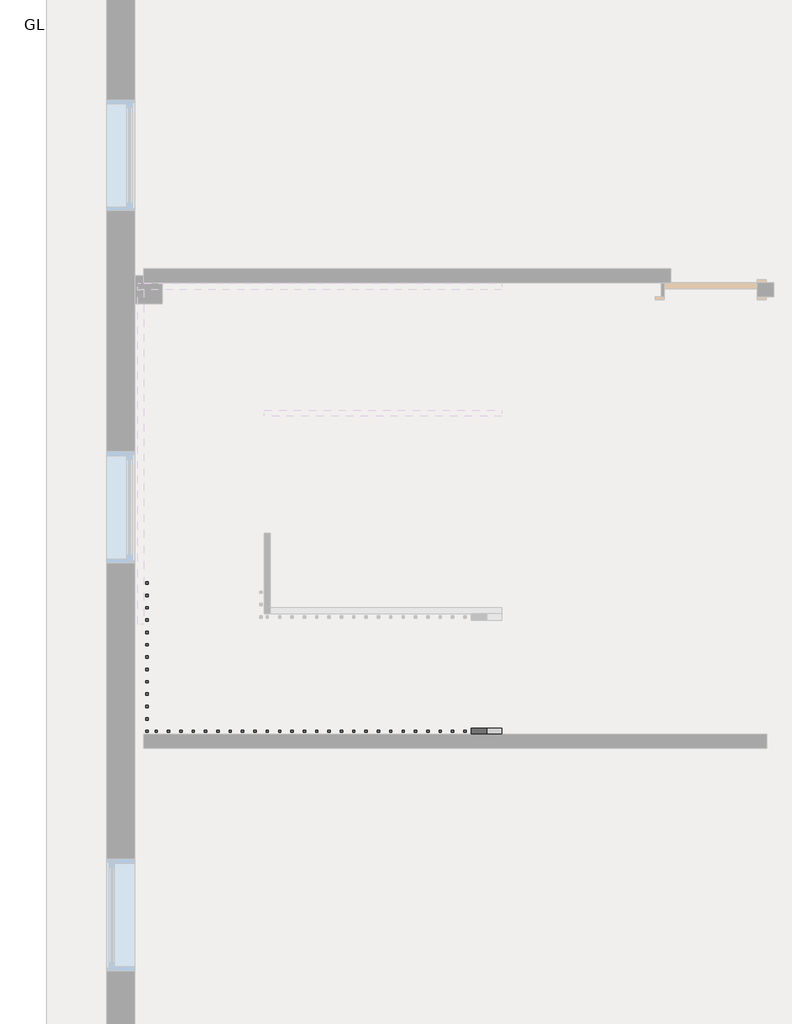
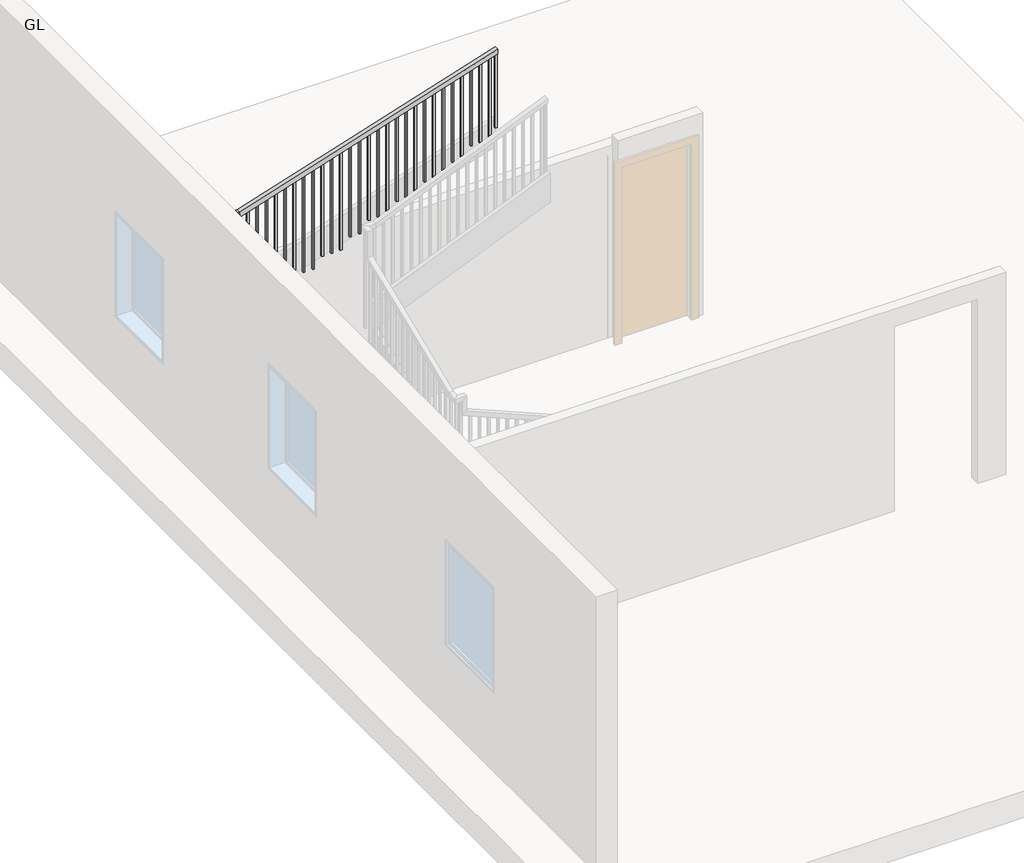
# One storey, part 2 of 3: 1 railing.
"""IFC4 building model written with IfcOpenShell, lengths in millimetres."""

from ifc_helpers import new_model, si_unit, frame, origin, place, context, project, spatial, polyline, outline, extrude, faceted_brep, element, save

model = new_model("IFC4")

# Units and contexts
model_context = context("Model", 3, world=origin())
ifc_project = project(units=[si_unit("LENGTHUNIT", "METRE", prefix="MILLI")], contexts=[model_context])

# Site, building, storey
site = spatial("IfcSite", under=ifc_project)
building = spatial("IfcBuilding", under=site)
storey = spatial("IfcBuildingStorey", under=building, Name="GL", Elevation=3200.4)

# Railing
placement = place(None, origin())
element("IfcRailing", 1, ObjectType="Handrail - Rectangular", at=placement, inside=storey, context=model_context, shape_type="SolidModel", body=[
    faceted_brep([(5202.3334712, 4110.8450307, 4349.2615385), (5202.3334712, 4110.8450307, 4294.1711054), (5202.3334712, 4161.6450307, 4294.1711054), (5202.3334712, 4161.6450307, 4349.2615385), (2978.1401378, 4110.8450307, 5282.4895105), (2967.9146058, 4110.8450307, 5231.6895105), (2967.9146058, 4161.6450307, 5231.6895105), (2978.1401378, 4161.6450307, 5282.4895105), (2255.9334712, 4110.8450307, 5231.6895105), (2255.9334712, 4110.8450307, 5282.4895105), (2255.9334712, 5086.4359398, 5282.4895105), (2255.9334712, 5094.0746153, 5231.6895105), (2306.7334712, 4161.6450307, 5231.6895105), (2306.7334712, 5094.0746153, 5231.6895105), (2306.7334712, 4161.6450307, 5282.4895105), (2306.7334712, 5086.4359398, 5282.4895105), (5202.3334712, 7768.4450307, 7045.5692308), (5202.3334712, 7717.6450307, 7045.5692308), (5202.3334712, 7717.6450307, 6992.2578701), (5202.3334712, 7768.4450307, 6992.2578701), (2390.8233294, 7768.4450307, 6097.3474801), (2382.9334712, 7768.4450307, 6148.1474801), (2390.8233294, 7717.6450307, 6097.3474801), (2382.9334712, 7717.6450307, 6148.1474801), (2255.9334712, 7641.4450307, 6068.6461538), (2255.9334712, 7692.2450307, 6031.1265614), (2306.7334712, 7692.2450307, 6031.1265614), (2306.7334712, 7641.4450307, 6068.6461538), (2255.9334712, 7641.4450307, 6148.1474801), (2255.9334712, 7692.2450307, 6097.3474801), (2306.7334712, 7692.2450307, 6097.3474801), (2306.7334712, 7641.4450307, 6148.1474801), (2255.9334712, 7768.4450307, 6148.1474801), (2255.9334712, 7768.4450307, 6097.3474801), (2306.7334712, 7717.6450307, 6097.3474801), (2306.7334712, 7717.6450307, 6148.1474801)], [[[0, 1, 2, 3]], [[1, 0, 4, 5]], [[2, 1, 5, 6]], [[3, 2, 6, 7]], [[0, 3, 7, 4]], [[8, 9, 10, 11]], [[12, 8, 11, 13]], [[14, 12, 13, 15]], [[9, 14, 15, 10]], [[16, 17, 18, 19]], [[20, 21, 16, 19]], [[22, 20, 19, 18]], [[23, 22, 18, 17]], [[21, 23, 17, 16]], [[5, 4, 9, 8]], [[6, 5, 8, 12]], [[7, 6, 12, 14]], [[4, 7, 14, 9]], [[11, 10, 24, 25]], [[13, 11, 25, 26]], [[15, 13, 26, 27]], [[10, 15, 27, 24]], [[25, 24, 28, 29]], [[26, 25, 29, 30]], [[27, 26, 30, 31]], [[24, 27, 31, 28]], [[29, 28, 32, 33]], [[30, 29, 33, 34]], [[31, 30, 34, 35]], [[28, 31, 35, 32]], [[33, 32, 21, 20]], [[34, 33, 20, 22]], [[35, 34, 22, 23]], [[32, 35, 23, 21]]]),
    extrude(outline(polyline([(6964.9713979, 5116.6084712), (6013.9384615, 5116.6084712), (6013.9384615, 5135.6584712), (6971.0350584, 5135.6584712), (6964.9713979, 5116.6084712)])), frame((0.0, 7733.5200307, 0.0), z_axis=(0.0, 1.0, 0.0), x_axis=(0.0, 0.0, 1.0)), (0.0, 0.0, 1.0), 19.05),
    extrude(outline(polyline([(6932.6318754, 5015.0084712), (6013.9384615, 5015.0084712), (6013.9384615, 5034.0584712), (6938.6955359, 5034.0584712), (6932.6318754, 5015.0084712)])), frame((0.0, 7733.5200307, 0.0), z_axis=(0.0, 1.0, 0.0), x_axis=(0.0, 0.0, 1.0)), (0.0, 0.0, 1.0), 19.05),
    extrude(outline(polyline([(6900.2923528, 4913.4084712), (6013.9384615, 4913.4084712), (6013.9384615, 4932.4584712), (6906.3560133, 4932.4584712), (6900.2923528, 4913.4084712)])), frame((0.0, 7733.5200307, 0.0), z_axis=(0.0, 1.0, 0.0), x_axis=(0.0, 0.0, 1.0)), (0.0, 0.0, 1.0), 19.05),
    extrude(outline(polyline([(6867.9528303, 4811.8084712), (5896.7076923, 4811.8084712), (5896.7076923, 4830.8584712), (6874.0164908, 4830.8584712), (6867.9528303, 4811.8084712)])), frame((0.0, 7733.5200307, 0.0), z_axis=(0.0, 1.0, 0.0), x_axis=(0.0, 0.0, 1.0)), (0.0, 0.0, 1.0), 19.05),
    extrude(outline(polyline([(6835.6133077, 4710.2084712), (5896.7076923, 4710.2084712), (5896.7076923, 4729.2584712), (6841.6769682, 4729.2584712), (6835.6133077, 4710.2084712)])), frame((0.0, 7733.5200307, 0.0), z_axis=(0.0, 1.0, 0.0), x_axis=(0.0, 0.0, 1.0)), (0.0, 0.0, 1.0), 19.05),
    extrude(outline(polyline([(6803.2737852, 4608.6084712), (5779.4769231, 4608.6084712), (5779.4769231, 4627.6584712), (6809.3374457, 4627.6584712), (6803.2737852, 4608.6084712)])), frame((0.0, 7733.5200307, 0.0), z_axis=(0.0, 1.0, 0.0), x_axis=(0.0, 0.0, 1.0)), (0.0, 0.0, 1.0), 19.05),
    extrude(outline(polyline([(6770.9342626, 4507.0084712), (5779.4769231, 4507.0084712), (5779.4769231, 4526.0584712), (6776.9979231, 4526.0584712), (6770.9342626, 4507.0084712)])), frame((0.0, 7733.5200307, 0.0), z_axis=(0.0, 1.0, 0.0), x_axis=(0.0, 0.0, 1.0)), (0.0, 0.0, 1.0), 19.05),
    extrude(outline(polyline([(6738.5947401, 4405.4084712), (5779.4769231, 4405.4084712), (5779.4769231, 4424.4584712), (6744.6584006, 4424.4584712), (6738.5947401, 4405.4084712)])), frame((0.0, 7733.5200307, 0.0), z_axis=(0.0, 1.0, 0.0), x_axis=(0.0, 0.0, 1.0)), (0.0, 0.0, 1.0), 19.05),
    extrude(outline(polyline([(6706.2552176, 4303.8084712), (5662.2461538, 4303.8084712), (5662.2461538, 4322.8584712), (6712.318878, 4322.8584712), (6706.2552176, 4303.8084712)])), frame((0.0, 7733.5200307, 0.0), z_axis=(0.0, 1.0, 0.0), x_axis=(0.0, 0.0, 1.0)), (0.0, 0.0, 1.0), 19.05),
    extrude(outline(polyline([(6673.915695, 4202.2084712), (5662.2461538, 4202.2084712), (5662.2461538, 4221.2584712), (6679.9793555, 4221.2584712), (6673.915695, 4202.2084712)])), frame((0.0, 7733.5200307, 0.0), z_axis=(0.0, 1.0, 0.0), x_axis=(0.0, 0.0, 1.0)), (0.0, 0.0, 1.0), 19.05),
    extrude(outline(polyline([(6641.5761725, 4100.6084712), (5662.2461538, 4100.6084712), (5662.2461538, 4119.6584712), (6647.6398329, 4119.6584712), (6641.5761725, 4100.6084712)])), frame((0.0, 7733.5200307, 0.0), z_axis=(0.0, 1.0, 0.0), x_axis=(0.0, 0.0, 1.0)), (0.0, 0.0, 1.0), 19.05),
    extrude(outline(polyline([(6609.2366499, 3999.0084712), (5545.0153846, 3999.0084712), (5545.0153846, 4018.0584712), (6615.3003104, 4018.0584712), (6609.2366499, 3999.0084712)])), frame((0.0, 7733.5200307, 0.0), z_axis=(0.0, 1.0, 0.0), x_axis=(0.0, 0.0, 1.0)), (0.0, 0.0, 1.0), 19.05),
    extrude(outline(polyline([(6576.8971274, 3897.4084712), (5545.0153846, 3897.4084712), (5545.0153846, 3916.4584712), (6582.9607878, 3916.4584712), (6576.8971274, 3897.4084712)])), frame((0.0, 7733.5200307, 0.0), z_axis=(0.0, 1.0, 0.0), x_axis=(0.0, 0.0, 1.0)), (0.0, 0.0, 1.0), 19.05),
    extrude(outline(polyline([(6544.5576048, 3795.8084712), (5545.0153846, 3795.8084712), (5545.0153846, 3814.8584712), (6550.6212653, 3814.8584712), (6544.5576048, 3795.8084712)])), frame((0.0, 7733.5200307, 0.0), z_axis=(0.0, 1.0, 0.0), x_axis=(0.0, 0.0, 1.0)), (0.0, 0.0, 1.0), 19.05),
    extrude(outline(polyline([(6512.2180823, 3694.2084712), (5427.7846154, 3694.2084712), (5427.7846154, 3713.2584712), (6518.2817427, 3713.2584712), (6512.2180823, 3694.2084712)])), frame((0.0, 7733.5200307, 0.0), z_axis=(0.0, 1.0, 0.0), x_axis=(0.0, 0.0, 1.0)), (0.0, 0.0, 1.0), 19.05),
    extrude(outline(polyline([(6479.8785597, 3592.6084712), (5427.7846154, 3592.6084712), (5427.7846154, 3611.6584712), (6485.9422202, 3611.6584712), (6479.8785597, 3592.6084712)])), frame((0.0, 7733.5200307, 0.0), z_axis=(0.0, 1.0, 0.0), x_axis=(0.0, 0.0, 1.0)), (0.0, 0.0, 1.0), 19.05),
    extrude(outline(polyline([(6447.5390372, 3491.0084712), (5310.5538462, 3491.0084712), (5310.5538462, 3510.0584712), (6453.6026977, 3510.0584712), (6447.5390372, 3491.0084712)])), frame((0.0, 7733.5200307, 0.0), z_axis=(0.0, 1.0, 0.0), x_axis=(0.0, 0.0, 1.0)), (0.0, 0.0, 1.0), 19.05),
    extrude(outline(polyline([(6415.1995146, 3389.4084712), (5310.5538462, 3389.4084712), (5310.5538462, 3408.4584712), (6421.2631751, 3408.4584712), (6415.1995146, 3389.4084712)])), frame((0.0, 7733.5200307, 0.0), z_axis=(0.0, 1.0, 0.0), x_axis=(0.0, 0.0, 1.0)), (0.0, 0.0, 1.0), 19.05),
    extrude(outline(polyline([(6382.8599921, 3287.8084712), (5310.5538462, 3287.8084712), (5310.5538462, 3306.8584712), (6388.9236526, 3306.8584712), (6382.8599921, 3287.8084712)])), frame((0.0, 7733.5200307, 0.0), z_axis=(0.0, 1.0, 0.0), x_axis=(0.0, 0.0, 1.0)), (0.0, 0.0, 1.0), 19.05),
    extrude(outline(polyline([(6350.5204695, 3186.2084712), (5193.3230769, 3186.2084712), (5193.3230769, 3205.2584712), (6356.58413, 3205.2584712), (6350.5204695, 3186.2084712)])), frame((0.0, 7733.5200307, 0.0), z_axis=(0.0, 1.0, 0.0), x_axis=(0.0, 0.0, 1.0)), (0.0, 0.0, 1.0), 19.05),
    extrude(outline(polyline([(6318.180947, 3084.6084712), (5193.3230769, 3084.6084712), (5193.3230769, 3103.6584712), (6324.2446075, 3103.6584712), (6318.180947, 3084.6084712)])), frame((0.0, 7733.5200307, 0.0), z_axis=(0.0, 1.0, 0.0), x_axis=(0.0, 0.0, 1.0)), (0.0, 0.0, 1.0), 19.05),
    extrude(outline(polyline([(6285.8414244, 2983.0084712), (5193.3230769, 2983.0084712), (5193.3230769, 3002.0584712), (6291.9050849, 3002.0584712), (6285.8414244, 2983.0084712)])), frame((0.0, 7733.5200307, 0.0), z_axis=(0.0, 1.0, 0.0), x_axis=(0.0, 0.0, 1.0)), (0.0, 0.0, 1.0), 19.05),
    extrude(outline(polyline([(6253.5019019, 2881.4084712), (5193.3230769, 2881.4084712), (5193.3230769, 2900.4584712), (6259.5655624, 2900.4584712), (6253.5019019, 2881.4084712)])), frame((0.0, 7733.5200307, 0.0), z_axis=(0.0, 1.0, 0.0), x_axis=(0.0, 0.0, 1.0)), (0.0, 0.0, 1.0), 19.05),
    extrude(outline(polyline([(6221.1623794, 2779.8084712), (5193.3230769, 2779.8084712), (5193.3230769, 2798.8584712), (6227.2260398, 2798.8584712), (6221.1623794, 2779.8084712)])), frame((0.0, 7733.5200307, 0.0), z_axis=(0.0, 1.0, 0.0), x_axis=(0.0, 0.0, 1.0)), (0.0, 0.0, 1.0), 19.05),
    extrude(outline(polyline([(6188.8228568, 2678.2084712), (5193.3230769, 2678.2084712), (5193.3230769, 2697.2584712), (6194.8865173, 2697.2584712), (6188.8228568, 2678.2084712)])), frame((0.0, 7733.5200307, 0.0), z_axis=(0.0, 1.0, 0.0), x_axis=(0.0, 0.0, 1.0)), (0.0, 0.0, 1.0), 19.05),
    extrude(outline(polyline([(6156.4833343, 2576.6084712), (5193.3230769, 2576.6084712), (5193.3230769, 2595.6584712), (6162.5469947, 2595.6584712), (6156.4833343, 2576.6084712)])), frame((0.0, 7733.5200307, 0.0), z_axis=(0.0, 1.0, 0.0), x_axis=(0.0, 0.0, 1.0)), (0.0, 0.0, 1.0), 19.05),
    extrude(outline(polyline([(6124.1438117, 2475.0084712), (5193.3230769, 2475.0084712), (5193.3230769, 2494.0584712), (6130.2074722, 2494.0584712), (6124.1438117, 2475.0084712)])), frame((0.0, 7733.5200307, 0.0), z_axis=(0.0, 1.0, 0.0), x_axis=(0.0, 0.0, 1.0)), (0.0, 0.0, 1.0), 19.05),
    extrude(outline(polyline([(6091.8042892, 2373.4084712), (5193.3230769, 2373.4084712), (5193.3230769, 2392.4584712), (6097.8679496, 2392.4584712), (6091.8042892, 2373.4084712)])), frame((0.0, 7733.5200307, 0.0), z_axis=(0.0, 1.0, 0.0), x_axis=(0.0, 0.0, 1.0)), (0.0, 0.0, 1.0), 19.05),
    extrude(outline(polyline([(2271.8084712, 7682.7200307), (2271.8084712, 7701.7700307), (2290.8584712, 7701.7700307), (2290.8584712, 7682.7200307), (2271.8084712, 7682.7200307)])), frame((0.0, 0.0, 5076.0923077), z_axis=(0.0, 0.0, 1.0), x_axis=(1.0, 0.0, 0.0)), (0.0, 0.0, 1.0), 1021.2551724),
    extrude(outline(polyline([(7600.1700307, 6002.7957922), (7600.1700307, 5076.0923077), (7581.1200307, 5076.0923077), (7581.1200307, 5996.9342537), (7600.1700307, 6002.7957922)])), frame((2271.8084712, 0.0, 0.0), z_axis=(1.0, 0.0, 0.0), x_axis=(0.0, 1.0, 0.0)), (0.0, 0.0, 1.0), 19.05),
    extrude(outline(polyline([(7498.5700307, 5971.5342537), (7498.5700307, 5076.0923077), (7479.5200307, 5076.0923077), (7479.5200307, 5965.6727152), (7498.5700307, 5971.5342537)])), frame((2271.8084712, 0.0, 0.0), z_axis=(1.0, 0.0, 0.0), x_axis=(0.0, 1.0, 0.0)), (0.0, 0.0, 1.0), 19.05),
    extrude(outline(polyline([(7396.9700307, 5940.2727152), (7396.9700307, 5076.0923077), (7377.9200307, 5076.0923077), (7377.9200307, 5934.4111768), (7396.9700307, 5940.2727152)])), frame((2271.8084712, 0.0, 0.0), z_axis=(1.0, 0.0, 0.0), x_axis=(0.0, 1.0, 0.0)), (0.0, 0.0, 1.0), 19.05),
    extrude(outline(polyline([(7295.3700307, 5909.0111768), (7295.3700307, 5076.0923077), (7276.3200307, 5076.0923077), (7276.3200307, 5903.1496383), (7295.3700307, 5909.0111768)])), frame((2271.8084712, 0.0, 0.0), z_axis=(1.0, 0.0, 0.0), x_axis=(0.0, 1.0, 0.0)), (0.0, 0.0, 1.0), 19.05),
    extrude(outline(polyline([(7193.7700307, 5877.7496383), (7193.7700307, 5076.0923077), (7174.7200307, 5076.0923077), (7174.7200307, 5871.8880999), (7193.7700307, 5877.7496383)])), frame((2271.8084712, 0.0, 0.0), z_axis=(1.0, 0.0, 0.0), x_axis=(0.0, 1.0, 0.0)), (0.0, 0.0, 1.0), 19.05),
    extrude(outline(polyline([(7092.1700307, 5846.4880999), (7092.1700307, 5076.0923077), (7073.1200307, 5076.0923077), (7073.1200307, 5840.6265614), (7092.1700307, 5846.4880999)])), frame((2271.8084712, 0.0, 0.0), z_axis=(1.0, 0.0, 0.0), x_axis=(0.0, 1.0, 0.0)), (0.0, 0.0, 1.0), 19.05),
    extrude(outline(polyline([(6990.5700307, 5815.2265614), (6990.5700307, 5076.0923077), (6971.5200307, 5076.0923077), (6971.5200307, 5809.3650229), (6990.5700307, 5815.2265614)])), frame((2271.8084712, 0.0, 0.0), z_axis=(1.0, 0.0, 0.0), x_axis=(0.0, 1.0, 0.0)), (0.0, 0.0, 1.0), 19.05),
    extrude(outline(polyline([(6888.9700307, 5783.9650229), (6888.9700307, 5076.0923077), (6869.9200307, 5076.0923077), (6869.9200307, 5778.1034845), (6888.9700307, 5783.9650229)])), frame((2271.8084712, 0.0, 0.0), z_axis=(1.0, 0.0, 0.0), x_axis=(0.0, 1.0, 0.0)), (0.0, 0.0, 1.0), 19.05),
    extrude(outline(polyline([(6787.3700307, 5752.7034845), (6787.3700307, 5076.0923077), (6768.3200307, 5076.0923077), (6768.3200307, 5746.841946), (6787.3700307, 5752.7034845)])), frame((2271.8084712, 0.0, 0.0), z_axis=(1.0, 0.0, 0.0), x_axis=(0.0, 1.0, 0.0)), (0.0, 0.0, 1.0), 19.05),
    extrude(outline(polyline([(6685.7700307, 5721.441946), (6685.7700307, 4958.8615385), (6666.7200307, 4958.8615385), (6666.7200307, 5715.5804076), (6685.7700307, 5721.441946)])), frame((2271.8084712, 0.0, 0.0), z_axis=(1.0, 0.0, 0.0), x_axis=(0.0, 1.0, 0.0)), (0.0, 0.0, 1.0), 19.05),
    extrude(outline(polyline([(6584.1700307, 5690.1804076), (6584.1700307, 4958.8615385), (6565.1200307, 4958.8615385), (6565.1200307, 5684.3188691), (6584.1700307, 5690.1804076)])), frame((2271.8084712, 0.0, 0.0), z_axis=(1.0, 0.0, 0.0), x_axis=(0.0, 1.0, 0.0)), (0.0, 0.0, 1.0), 19.05),
    extrude(outline(polyline([(6482.5700307, 5658.9188691), (6482.5700307, 4841.6307692), (6463.5200307, 4841.6307692), (6463.5200307, 5653.0573306), (6482.5700307, 5658.9188691)])), frame((2271.8084712, 0.0, 0.0), z_axis=(1.0, 0.0, 0.0), x_axis=(0.0, 1.0, 0.0)), (0.0, 0.0, 1.0), 19.05),
    extrude(outline(polyline([(6380.9700307, 5627.6573306), (6380.9700307, 4841.6307692), (6361.9200307, 4841.6307692), (6361.9200307, 5621.7957922), (6380.9700307, 5627.6573306)])), frame((2271.8084712, 0.0, 0.0), z_axis=(1.0, 0.0, 0.0), x_axis=(0.0, 1.0, 0.0)), (0.0, 0.0, 1.0), 19.05),
    extrude(outline(polyline([(6279.3700307, 5596.3957922), (6279.3700307, 4841.6307692), (6260.3200307, 4841.6307692), (6260.3200307, 5590.5342537), (6279.3700307, 5596.3957922)])), frame((2271.8084712, 0.0, 0.0), z_axis=(1.0, 0.0, 0.0), x_axis=(0.0, 1.0, 0.0)), (0.0, 0.0, 1.0), 19.05),
    extrude(outline(polyline([(6177.7700307, 5565.1342537), (6177.7700307, 4724.4), (6158.7200307, 4724.4), (6158.7200307, 5559.2727152), (6177.7700307, 5565.1342537)])), frame((2271.8084712, 0.0, 0.0), z_axis=(1.0, 0.0, 0.0), x_axis=(0.0, 1.0, 0.0)), (0.0, 0.0, 1.0), 19.05),
    extrude(outline(polyline([(6076.1700307, 5533.8727152), (6076.1700307, 4724.4), (6057.1200307, 4724.4), (6057.1200307, 5528.0111768), (6076.1700307, 5533.8727152)])), frame((2271.8084712, 0.0, 0.0), z_axis=(1.0, 0.0, 0.0), x_axis=(0.0, 1.0, 0.0)), (0.0, 0.0, 1.0), 19.05),
    extrude(outline(polyline([(5974.5700307, 5502.6111768), (5974.5700307, 4724.4), (5955.5200307, 4724.4), (5955.5200307, 5496.7496383), (5974.5700307, 5502.6111768)])), frame((2271.8084712, 0.0, 0.0), z_axis=(1.0, 0.0, 0.0), x_axis=(0.0, 1.0, 0.0)), (0.0, 0.0, 1.0), 19.05),
    extrude(outline(polyline([(5872.9700307, 5471.3496383), (5872.9700307, 4607.1692308), (5853.9200307, 4607.1692308), (5853.9200307, 5465.4880999), (5872.9700307, 5471.3496383)])), frame((2271.8084712, 0.0, 0.0), z_axis=(1.0, 0.0, 0.0), x_axis=(0.0, 1.0, 0.0)), (0.0, 0.0, 1.0), 19.05),
    extrude(outline(polyline([(5771.3700307, 5440.0880999), (5771.3700307, 4607.1692308), (5752.3200307, 4607.1692308), (5752.3200307, 5434.2265614), (5771.3700307, 5440.0880999)])), frame((2271.8084712, 0.0, 0.0), z_axis=(1.0, 0.0, 0.0), x_axis=(0.0, 1.0, 0.0)), (0.0, 0.0, 1.0), 19.05),
    extrude(outline(polyline([(5669.7700307, 5408.8265614), (5669.7700307, 4607.1692308), (5650.7200307, 4607.1692308), (5650.7200307, 5402.9650229), (5669.7700307, 5408.8265614)])), frame((2271.8084712, 0.0, 0.0), z_axis=(1.0, 0.0, 0.0), x_axis=(0.0, 1.0, 0.0)), (0.0, 0.0, 1.0), 19.05),
    extrude(outline(polyline([(5568.1700307, 5377.5650229), (5568.1700307, 4489.9384615), (5549.1200307, 4489.9384615), (5549.1200307, 5371.7034845), (5568.1700307, 5377.5650229)])), frame((2271.8084712, 0.0, 0.0), z_axis=(1.0, 0.0, 0.0), x_axis=(0.0, 1.0, 0.0)), (0.0, 0.0, 1.0), 19.05),
    extrude(outline(polyline([(5466.5700307, 5346.3034845), (5466.5700307, 4489.9384615), (5447.5200307, 4489.9384615), (5447.5200307, 5340.441946), (5466.5700307, 5346.3034845)])), frame((2271.8084712, 0.0, 0.0), z_axis=(1.0, 0.0, 0.0), x_axis=(0.0, 1.0, 0.0)), (0.0, 0.0, 1.0), 19.05),
    extrude(outline(polyline([(5364.9700307, 5315.041946), (5364.9700307, 4372.7076923), (5345.9200307, 4372.7076923), (5345.9200307, 5309.1804076), (5364.9700307, 5315.041946)])), frame((2271.8084712, 0.0, 0.0), z_axis=(1.0, 0.0, 0.0), x_axis=(0.0, 1.0, 0.0)), (0.0, 0.0, 1.0), 19.05),
    extrude(outline(polyline([(5263.3700307, 5283.7804076), (5263.3700307, 4372.7076923), (5244.3200307, 4372.7076923), (5244.3200307, 5277.9188691), (5263.3700307, 5283.7804076)])), frame((2271.8084712, 0.0, 0.0), z_axis=(1.0, 0.0, 0.0), x_axis=(0.0, 1.0, 0.0)), (0.0, 0.0, 1.0), 19.05),
    extrude(outline(polyline([(5161.7700307, 5252.5188691), (5161.7700307, 4372.7076923), (5142.7200307, 4372.7076923), (5142.7200307, 5246.6573306), (5161.7700307, 5252.5188691)])), frame((2271.8084712, 0.0, 0.0), z_axis=(1.0, 0.0, 0.0), x_axis=(0.0, 1.0, 0.0)), (0.0, 0.0, 1.0), 19.05),
    extrude(outline(polyline([(2271.8084712, 5041.1200307), (2271.8084712, 5060.1700307), (2290.8584712, 5060.1700307), (2290.8584712, 5041.1200307), (2271.8084712, 5041.1200307)])), frame((0.0, 0.0, 4255.4769231), z_axis=(0.0, 0.0, 1.0), x_axis=(1.0, 0.0, 0.0)), (0.0, 0.0, 1.0), 976.2125874),
    extrude(outline(polyline([(2271.8084712, 4939.5200307), (2271.8084712, 4958.5700307), (2290.8584712, 4958.5700307), (2290.8584712, 4939.5200307), (2271.8084712, 4939.5200307)])), frame((0.0, 0.0, 4255.4769231), z_axis=(0.0, 0.0, 1.0), x_axis=(1.0, 0.0, 0.0)), (0.0, 0.0, 1.0), 976.2125874),
    extrude(outline(polyline([(2271.8084712, 4837.9200307), (2271.8084712, 4856.9700307), (2290.8584712, 4856.9700307), (2290.8584712, 4837.9200307), (2271.8084712, 4837.9200307)])), frame((0.0, 0.0, 4255.4769231), z_axis=(0.0, 0.0, 1.0), x_axis=(1.0, 0.0, 0.0)), (0.0, 0.0, 1.0), 976.2125874),
    extrude(outline(polyline([(2271.8084712, 4736.3200307), (2271.8084712, 4755.3700307), (2290.8584712, 4755.3700307), (2290.8584712, 4736.3200307), (2271.8084712, 4736.3200307)])), frame((0.0, 0.0, 4255.4769231), z_axis=(0.0, 0.0, 1.0), x_axis=(1.0, 0.0, 0.0)), (0.0, 0.0, 1.0), 976.2125874),
    extrude(outline(polyline([(2271.8084712, 4634.7200307), (2271.8084712, 4653.7700307), (2290.8584712, 4653.7700307), (2290.8584712, 4634.7200307), (2271.8084712, 4634.7200307)])), frame((0.0, 0.0, 4255.4769231), z_axis=(0.0, 0.0, 1.0), x_axis=(1.0, 0.0, 0.0)), (0.0, 0.0, 1.0), 976.2125874),
    extrude(outline(polyline([(2271.8084712, 4533.1200307), (2271.8084712, 4552.1700307), (2290.8584712, 4552.1700307), (2290.8584712, 4533.1200307), (2271.8084712, 4533.1200307)])), frame((0.0, 0.0, 4255.4769231), z_axis=(0.0, 0.0, 1.0), x_axis=(1.0, 0.0, 0.0)), (0.0, 0.0, 1.0), 976.2125874),
    extrude(outline(polyline([(2271.8084712, 4431.5200307), (2271.8084712, 4450.5700307), (2290.8584712, 4450.5700307), (2290.8584712, 4431.5200307), (2271.8084712, 4431.5200307)])), frame((0.0, 0.0, 4255.4769231), z_axis=(0.0, 0.0, 1.0), x_axis=(1.0, 0.0, 0.0)), (0.0, 0.0, 1.0), 976.2125874),
    extrude(outline(polyline([(2271.8084712, 4329.9200307), (2271.8084712, 4348.9700307), (2290.8584712, 4348.9700307), (2290.8584712, 4329.9200307), (2271.8084712, 4329.9200307)])), frame((0.0, 0.0, 4255.4769231), z_axis=(0.0, 0.0, 1.0), x_axis=(1.0, 0.0, 0.0)), (0.0, 0.0, 1.0), 976.2125874),
    extrude(outline(polyline([(2271.8084712, 4228.3200307), (2271.8084712, 4247.3700307), (2290.8584712, 4247.3700307), (2290.8584712, 4228.3200307), (2271.8084712, 4228.3200307)])), frame((0.0, 0.0, 4255.4769231), z_axis=(0.0, 0.0, 1.0), x_axis=(1.0, 0.0, 0.0)), (0.0, 0.0, 1.0), 976.2125874),
    extrude(outline(polyline([(2367.0584712, 4126.7200307), (2348.0084712, 4126.7200307), (2348.0084712, 4145.7700307), (2367.0584712, 4145.7700307), (2367.0584712, 4126.7200307)])), frame((0.0, 0.0, 4255.4769231), z_axis=(0.0, 0.0, 1.0), x_axis=(1.0, 0.0, 0.0)), (0.0, 0.0, 1.0), 976.2125874),
    extrude(outline(polyline([(2468.6584712, 4126.7200307), (2449.6084712, 4126.7200307), (2449.6084712, 4145.7700307), (2468.6584712, 4145.7700307), (2468.6584712, 4126.7200307)])), frame((0.0, 0.0, 4255.4769231), z_axis=(0.0, 0.0, 1.0), x_axis=(1.0, 0.0, 0.0)), (0.0, 0.0, 1.0), 976.2125874),
    extrude(outline(polyline([(2570.2584712, 4126.7200307), (2551.2084712, 4126.7200307), (2551.2084712, 4145.7700307), (2570.2584712, 4145.7700307), (2570.2584712, 4126.7200307)])), frame((0.0, 0.0, 4255.4769231), z_axis=(0.0, 0.0, 1.0), x_axis=(1.0, 0.0, 0.0)), (0.0, 0.0, 1.0), 976.2125874),
    extrude(outline(polyline([(2671.8584712, 4126.7200307), (2652.8084712, 4126.7200307), (2652.8084712, 4145.7700307), (2671.8584712, 4145.7700307), (2671.8584712, 4126.7200307)])), frame((0.0, 0.0, 4255.4769231), z_axis=(0.0, 0.0, 1.0), x_axis=(1.0, 0.0, 0.0)), (0.0, 0.0, 1.0), 976.2125874),
    extrude(outline(polyline([(2773.4584712, 4126.7200307), (2754.4084712, 4126.7200307), (2754.4084712, 4145.7700307), (2773.4584712, 4145.7700307), (2773.4584712, 4126.7200307)])), frame((0.0, 0.0, 4255.4769231), z_axis=(0.0, 0.0, 1.0), x_axis=(1.0, 0.0, 0.0)), (0.0, 0.0, 1.0), 976.2125874),
    extrude(outline(polyline([(2875.0584712, 4126.7200307), (2856.0084712, 4126.7200307), (2856.0084712, 4145.7700307), (2875.0584712, 4145.7700307), (2875.0584712, 4126.7200307)])), frame((0.0, 0.0, 4255.4769231), z_axis=(0.0, 0.0, 1.0), x_axis=(1.0, 0.0, 0.0)), (0.0, 0.0, 1.0), 976.2125874),
    extrude(outline(polyline([(2976.6584712, 4126.7200307), (2957.6084712, 4126.7200307), (2957.6084712, 4145.7700307), (2976.6584712, 4145.7700307), (2976.6584712, 4126.7200307)])), frame((0.0, 0.0, 4255.4769231), z_axis=(0.0, 0.0, 1.0), x_axis=(1.0, 0.0, 0.0)), (0.0, 0.0, 1.0), 976.2125874),
    extrude(outline(polyline([(5193.3843922, 3059.2084712), (4255.4769231, 3059.2084712), (4255.4769231, 3078.2584712), (5185.3913852, 3078.2584712), (5193.3843922, 3059.2084712)])), frame((0.0, 4126.7200307, 0.0), z_axis=(0.0, 1.0, 0.0), x_axis=(0.0, 0.0, 1.0)), (0.0, 0.0, 1.0), 19.05),
    extrude(outline(polyline([(5150.7550215, 3160.8084712), (4255.4769231, 3160.8084712), (4255.4769231, 3179.8584712), (5142.7620145, 3179.8584712), (5150.7550215, 3160.8084712)])), frame((0.0, 4126.7200307, 0.0), z_axis=(0.0, 1.0, 0.0), x_axis=(0.0, 0.0, 1.0)), (0.0, 0.0, 1.0), 19.05),
    extrude(outline(polyline([(5108.1256509, 3262.4084712), (4138.2461538, 3262.4084712), (4138.2461538, 3281.4584712), (5100.1326439, 3281.4584712), (5108.1256509, 3262.4084712)])), frame((0.0, 4126.7200307, 0.0), z_axis=(0.0, 1.0, 0.0), x_axis=(0.0, 0.0, 1.0)), (0.0, 0.0, 1.0), 19.05),
    extrude(outline(polyline([(5065.4962803, 3364.0084712), (4138.2461538, 3364.0084712), (4138.2461538, 3383.0584712), (5057.5032733, 3383.0584712), (5065.4962803, 3364.0084712)])), frame((0.0, 4126.7200307, 0.0), z_axis=(0.0, 1.0, 0.0), x_axis=(0.0, 0.0, 1.0)), (0.0, 0.0, 1.0), 19.05),
    extrude(outline(polyline([(5022.8669096, 3465.6084712), (4138.2461538, 3465.6084712), (4138.2461538, 3484.6584712), (5014.8739026, 3484.6584712), (5022.8669096, 3465.6084712)])), frame((0.0, 4126.7200307, 0.0), z_axis=(0.0, 1.0, 0.0), x_axis=(0.0, 0.0, 1.0)), (0.0, 0.0, 1.0), 19.05),
    extrude(outline(polyline([(4980.237539, 3567.2084712), (4021.0153846, 3567.2084712), (4021.0153846, 3586.2584712), (4972.244532, 3586.2584712), (4980.237539, 3567.2084712)])), frame((0.0, 4126.7200307, 0.0), z_axis=(0.0, 1.0, 0.0), x_axis=(0.0, 0.0, 1.0)), (0.0, 0.0, 1.0), 19.05),
    extrude(outline(polyline([(4937.6081684, 3668.8084712), (4021.0153846, 3668.8084712), (4021.0153846, 3687.8584712), (4929.6151614, 3687.8584712), (4937.6081684, 3668.8084712)])), frame((0.0, 4126.7200307, 0.0), z_axis=(0.0, 1.0, 0.0), x_axis=(0.0, 0.0, 1.0)), (0.0, 0.0, 1.0), 19.05),
    extrude(outline(polyline([(4894.9787978, 3770.4084712), (4021.0153846, 3770.4084712), (4021.0153846, 3789.4584712), (4886.9857908, 3789.4584712), (4894.9787978, 3770.4084712)])), frame((0.0, 4126.7200307, 0.0), z_axis=(0.0, 1.0, 0.0), x_axis=(0.0, 0.0, 1.0)), (0.0, 0.0, 1.0), 19.05),
    extrude(outline(polyline([(4852.3494271, 3872.0084712), (3903.7846154, 3872.0084712), (3903.7846154, 3891.0584712), (4844.3564201, 3891.0584712), (4852.3494271, 3872.0084712)])), frame((0.0, 4126.7200307, 0.0), z_axis=(0.0, 1.0, 0.0), x_axis=(0.0, 0.0, 1.0)), (0.0, 0.0, 1.0), 19.05),
    extrude(outline(polyline([(4809.7200565, 3973.6084712), (3903.7846154, 3973.6084712), (3903.7846154, 3992.6584712), (4801.7270495, 3992.6584712), (4809.7200565, 3973.6084712)])), frame((0.0, 4126.7200307, 0.0), z_axis=(0.0, 1.0, 0.0), x_axis=(0.0, 0.0, 1.0)), (0.0, 0.0, 1.0), 19.05),
    extrude(outline(polyline([(4767.0906859, 4075.2084712), (3903.7846154, 4075.2084712), (3903.7846154, 4094.2584712), (4759.0976789, 4094.2584712), (4767.0906859, 4075.2084712)])), frame((0.0, 4126.7200307, 0.0), z_axis=(0.0, 1.0, 0.0), x_axis=(0.0, 0.0, 1.0)), (0.0, 0.0, 1.0), 19.05),
    extrude(outline(polyline([(4724.4613152, 4176.8084712), (3786.5538462, 4176.8084712), (3786.5538462, 4195.8584712), (4716.4683082, 4195.8584712), (4724.4613152, 4176.8084712)])), frame((0.0, 4126.7200307, 0.0), z_axis=(0.0, 1.0, 0.0), x_axis=(0.0, 0.0, 1.0)), (0.0, 0.0, 1.0), 19.05),
    extrude(outline(polyline([(4681.8319446, 4278.4084712), (3786.5538462, 4278.4084712), (3786.5538462, 4297.4584712), (4673.8389376, 4297.4584712), (4681.8319446, 4278.4084712)])), frame((0.0, 4126.7200307, 0.0), z_axis=(0.0, 1.0, 0.0), x_axis=(0.0, 0.0, 1.0)), (0.0, 0.0, 1.0), 19.05),
    extrude(outline(polyline([(4639.202574, 4380.0084712), (3669.3230769, 4380.0084712), (3669.3230769, 4399.0584712), (4631.209567, 4399.0584712), (4639.202574, 4380.0084712)])), frame((0.0, 4126.7200307, 0.0), z_axis=(0.0, 1.0, 0.0), x_axis=(0.0, 0.0, 1.0)), (0.0, 0.0, 1.0), 19.05),
    extrude(outline(polyline([(4596.5732033, 4481.6084712), (3669.3230769, 4481.6084712), (3669.3230769, 4500.6584712), (4588.5801964, 4500.6584712), (4596.5732033, 4481.6084712)])), frame((0.0, 4126.7200307, 0.0), z_axis=(0.0, 1.0, 0.0), x_axis=(0.0, 0.0, 1.0)), (0.0, 0.0, 1.0), 19.05),
    extrude(outline(polyline([(4553.9438327, 4583.2084712), (3669.3230769, 4583.2084712), (3669.3230769, 4602.2584712), (4545.9508257, 4602.2584712), (4553.9438327, 4583.2084712)])), frame((0.0, 4126.7200307, 0.0), z_axis=(0.0, 1.0, 0.0), x_axis=(0.0, 0.0, 1.0)), (0.0, 0.0, 1.0), 19.05),
    extrude(outline(polyline([(4511.3144621, 4684.8084712), (3552.0923077, 4684.8084712), (3552.0923077, 4703.8584712), (4503.3214551, 4703.8584712), (4511.3144621, 4684.8084712)])), frame((0.0, 4126.7200307, 0.0), z_axis=(0.0, 1.0, 0.0), x_axis=(0.0, 0.0, 1.0)), (0.0, 0.0, 1.0), 19.05),
    extrude(outline(polyline([(4468.6850915, 4786.4084712), (3552.0923077, 4786.4084712), (3552.0923077, 4805.4584712), (4460.6920845, 4805.4584712), (4468.6850915, 4786.4084712)])), frame((0.0, 4126.7200307, 0.0), z_axis=(0.0, 1.0, 0.0), x_axis=(0.0, 0.0, 1.0)), (0.0, 0.0, 1.0), 19.05),
    extrude(outline(polyline([(4426.0557208, 4888.0084712), (3552.0923077, 4888.0084712), (3552.0923077, 4907.0584712), (4418.0627138, 4907.0584712), (4426.0557208, 4888.0084712)])), frame((0.0, 4126.7200307, 0.0), z_axis=(0.0, 1.0, 0.0), x_axis=(0.0, 0.0, 1.0)), (0.0, 0.0, 1.0), 19.05),
    extrude(outline(polyline([(4383.4263502, 4989.6084712), (3434.8615385, 4989.6084712), (3434.8615385, 5008.6584712), (4375.4333432, 5008.6584712), (4383.4263502, 4989.6084712)])), frame((0.0, 4126.7200307, 0.0), z_axis=(0.0, 1.0, 0.0), x_axis=(0.0, 0.0, 1.0)), (0.0, 0.0, 1.0), 19.05),
    extrude(outline(polyline([(4340.7969796, 5091.2084712), (3434.8615385, 5091.2084712), (3434.8615385, 5110.2584712), (4332.8039726, 5110.2584712), (4340.7969796, 5091.2084712)])), frame((0.0, 4126.7200307, 0.0), z_axis=(0.0, 1.0, 0.0), x_axis=(0.0, 0.0, 1.0)), (0.0, 0.0, 1.0), 19.05),
    extrude(outline(polyline([(2271.8084712, 7733.5200307), (2271.8084712, 7752.5700307), (2290.8584712, 7752.5700307), (2290.8584712, 7733.5200307), (2271.8084712, 7733.5200307)])), frame((0.0, 0.0, 5076.0923077), z_axis=(0.0, 0.0, 1.0), x_axis=(1.0, 0.0, 0.0)), (0.0, 0.0, 1.0), 1021.2551724),
    extrude(outline(polyline([(2290.8584712, 4126.7200307), (2271.8084712, 4126.7200307), (2271.8084712, 4145.7700307), (2290.8584712, 4145.7700307), (2290.8584712, 4126.7200307)])), frame((0.0, 0.0, 4255.4769231), z_axis=(0.0, 0.0, 1.0), x_axis=(1.0, 0.0, 0.0)), (0.0, 0.0, 1.0), 976.2125874),
    extrude(outline(polyline([(6986.1942096, 5183.2834712), (6131.1692308, 5183.2834712), (6131.1692308, 5202.3334712), (6992.2578701, 5202.3334712), (6986.1942096, 5183.2834712)])), frame((0.0, 7733.5200307, 0.0), z_axis=(0.0, 1.0, 0.0), x_axis=(0.0, 0.0, 1.0)), (0.0, 0.0, 1.0), 19.05),
    extrude(outline(polyline([(4302.1641124, 5183.2834712), (3317.6307692, 5183.2834712), (3317.6307692, 5202.3334712), (4294.1711054, 5202.3334712), (4302.1641124, 5183.2834712)])), frame((0.0, 4126.7200307, 0.0), z_axis=(0.0, 1.0, 0.0), x_axis=(0.0, 0.0, 1.0)), (0.0, 0.0, 1.0), 19.05),
])

save(model, "model.ifc")

# Revit data of these elements
# Type "Handrail - Rectangular"
#   Assembly Code = "C2010400"
#   built-in parameter 1008612 = 0.0416667 (stored number, unit not read)
#   built-in parameter 1008611 = 0.0416667 (stored number, unit not read)
#   built-in parameter 1008609 = 0.333333 (stored number, unit not read)
#   built-in parameter 1008604 = 0.166667 (stored number, unit not read)
#   built-in parameter 1008603 = 0.166667 (stored number, unit not read)
#   Railing Height = 3' - 0"
#   built-in parameter 1008630 = 2
#   built-in parameter 1008610 = 2
#   built-in parameter 1008618 = Baluster - Square : 3/4"
# Element 1 (IfcRailing, "Handrail - Rectangular")
#   Phase Created = New Construction
